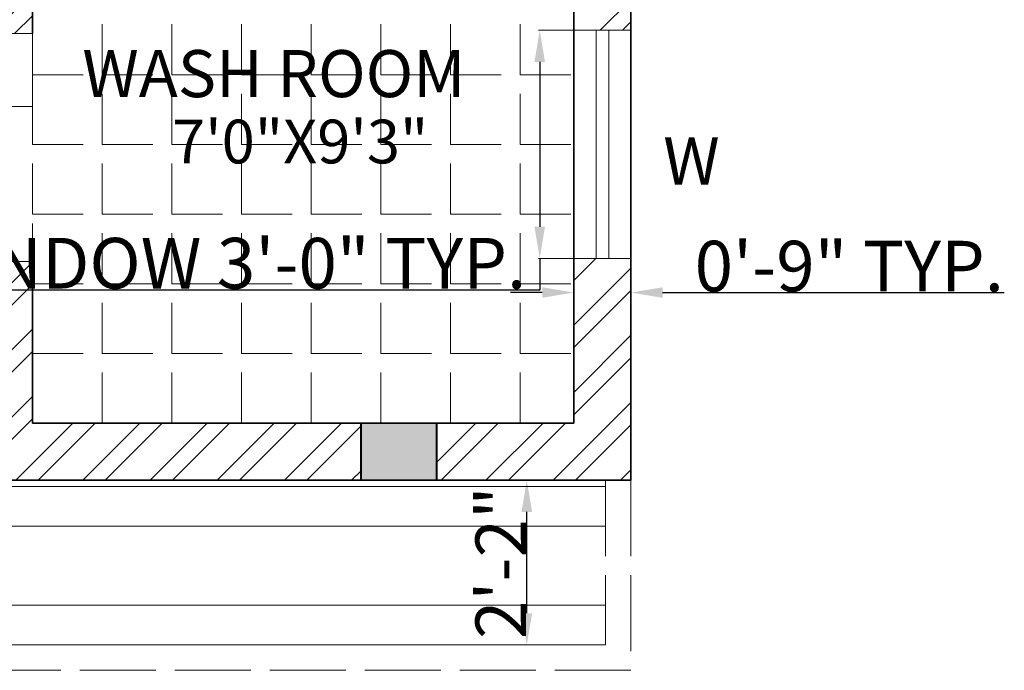
# Model space of a CAD drawing. Units: inches. Extents: x 351 to 1738, y -265 to 286.
# Tile 30 of 38: x 1470 to 1626, y -203 to -100. Entities that reach past the tile are written whole.
import ezdxf

# ---------------------------------------------------------------- set-up
doc = ezdxf.new("R2010")
doc.units = ezdxf.units.IN
doc.header["$MEASUREMENT"] = 0
doc.linetypes.add('ACAD_ISO02W100', pattern=[15, 12, -3])
doc.linetypes.add('ACAD_ISO03W100', pattern=[30, 12, -18])
for name, color, linetype, lineweight in [('A-ANNO-DIMS', 2, 'Continuous', 18), ('A-ANNO-SYMB', 7, 'Continuous', 18), ('A-AREA-IDEN', 7, 'Continuous', 18), ('A-COLS', 7, 'Continuous', 40), ('A-COLS-PATT', 6, 'Continuous', 13), ('A-DOOR', 3, 'Continuous', 18), ('A-DOOR-HIDN', 3, 'ACAD_ISO03W100', 13), ('A-FLOR-OVHD', 1, 'ACAD_ISO02W100', 18), ('A-FLOR-PATT', 9, 'Continuous', 9), ('A-GLAZ', 4, 'Continuous', 18), ('A-WALL', 7, 'Continuous', 35), ('A-WALL-PATT', 152, 'Continuous', 13)]:
    doc.layers.add(name, color=color, linetype=linetype, lineweight=lineweight)
doc.styles.add('Annotative', font='arial.ttf')
doc.styles.get("Standard").update_dxf_attribs({"font": 'arial.ttf'})
doc.dimstyles.get("Standard").update_dxf_attribs({"dimtxt": 8, "dimasz": 5, "dimexe": 0.18, "dimexo": 0.0625, "dimgap": 0.09, "dimtad": 1, "dimtoh": 1, "dimzin": 0, "dimdsep": 46, "dimlunit": 4, "dimtxsty": 'Standard', "dimcen": 0, "dimclre": 256, "dimadec": 0, "dimazin": 0, "dimtfac": 1, "dimtofl": 0, "dimtmove": 0, "dimatfit": 3, "dimfxl": 1, "dimtolj": 1, "dimtzin": 0, "dimlwe": -1, "dimarcsym": 0})

# ---------------------------------------------------------------- blocks, each defined once
blk = doc.blocks.new('*D10')
at = {"layer": 'A-ANNO-DIMS', "color": 0, "transparency": 16777216}
for p, q in [((1562.64, -173.04), (1550.08, -173.04)), ((1562.64, -199.04), (1550.08, -199.04))]:
    blk.add_line(p, q, dxfattribs=at)
at = {"layer": 'A-ANNO-DIMS', "color": 0, "lineweight": -2, "transparency": 16777216}
blk.add_line((1550.26, -194.04), (1550.26, -178.04), dxfattribs=at)
at = {"layer": 'A-ANNO-DIMS', "color": 0, "transparency": 16777216}
for points in [[(1549.43, -178.04), (1551.1, -178.04), (1550.26, -173.04)], [(1549.43, -194.04), (1551.1, -194.04), (1550.26, -199.04)]]:
    blk.add_solid(points, dxfattribs=at)
at = {"layer": 'Defpoints', "color": 0, "transparency": 16777216}
for p in [(1550.26, -173.04), (1562.7, -173.04), (1562.7, -199.04)]:
    blk.add_point(p, dxfattribs=at)
at = {"layer": 'A-ANNO-DIMS', "color": 0, "transparency": 16777216, "insert": (1546.16, -186.04), "char_height": 8, "attachment_point": 5, "rotation": 90}
blk.add_mtext('\\A1;2\'-2"', dxfattribs=at)
blk = doc.blocks.new('WIN-36')
for p, q in [((0, 5.5), (36, 5.5)), ((0, 3.5), (36, 3.5))]:
    blk.add_line(p, q)
blk.add_lwpolyline([(0, 9), (36, 9), (36, 0), (0, 0)], close=True)
blk = doc.blocks.new('*D32')
at = {"layer": 'A-ANNO-DIMS', "transparency": 16777216}
for p, q in [((1557.64, -102), (1552.12, -102)), ((1557.64, -138), (1552.12, -138))]:
    blk.add_line(p, q, dxfattribs=at)
at = {"layer": 'A-ANNO-DIMS', "color": 0, "lineweight": -2, "transparency": 16777216}
for p, q in [((1552.3, -107), (1552.3, -133)), ((1552.3, -138), (1552.3, -143)), ((1552.3, -143), (1450.98, -143))]:
    blk.add_line(p, q, dxfattribs=at)
at = {"layer": 'A-ANNO-DIMS', "color": 0, "transparency": 16777216}
for points in [[(1551.47, -107), (1553.14, -107), (1552.3, -102)], [(1551.47, -133), (1553.14, -133), (1552.3, -138)]]:
    blk.add_solid(points, dxfattribs=at)
at = {"layer": 'Defpoints', "color": 0, "transparency": 16777216}
for p in [(1557.7, -102), (1552.3, -138), (1557.7, -138)]:
    blk.add_point(p, dxfattribs=at)
at = {"layer": 'A-ANNO-DIMS', "color": 0, "transparency": 16777216, "insert": (1501.6, -138.77), "char_height": 8, "attachment_point": 5}
blk.add_mtext('\\A1;WINDOW 3\'-0" TYP.', dxfattribs=at)
blk = doc.blocks.new('*D33')
at = {"layer": 'A-ANNO-DIMS', "transparency": 16777216}
for p, q in [((1557.7, -138.06), (1557.7, -143.58)), ((1566.7, -138.06), (1566.7, -143.58))]:
    blk.add_line(p, q, dxfattribs=at)
at = {"layer": 'A-ANNO-DIMS', "color": 0, "lineweight": -2, "transparency": 16777216}
for p, q in [((1552.7, -143.4), (1547.7, -143.4)), ((1571.7, -143.4), (1625.65, -143.4))]:
    blk.add_line(p, q, dxfattribs=at)
at = {"layer": 'A-ANNO-DIMS', "color": 0, "transparency": 16777216}
for points in [[(1552.7, -142.57), (1552.7, -144.23), (1557.7, -143.4)], [(1571.7, -142.57), (1571.7, -144.23), (1566.7, -143.4)]]:
    blk.add_solid(points, dxfattribs=at)
at = {"layer": 'Defpoints', "color": 0, "transparency": 16777216}
for p in [(1557.7, -138), (1566.7, -138), (1566.7, -143.4)]:
    blk.add_point(p, dxfattribs=at)
at = {"layer": 'A-ANNO-DIMS', "color": 0, "transparency": 16777216, "insert": (1601.18, -139.23), "char_height": 8, "attachment_point": 5}
blk.add_mtext('\\A1;0\'-9" TYP.', dxfattribs=at)

msp = doc.modelspace()

# ---------------------------------------------------------------- hatches: boundary and pattern name
at = {"layer": 'A-COLS-PATT'}
h = msp.add_hatch(color=256, dxfattribs=at)
h.dxf.hatch_style = 1
h.paths.add_polyline_path([(1112.704, 237.963), (1103.704, 237.963), (1103.704, 228.963), (1112.704, 228.963)])
h.paths.add_polyline_path([(1115.704, 237.963), (1112.704, 237.963), (1112.704, 228.963), (1115.704, 228.963)])
h.paths.add_polyline_path([(1043.704, 255.963), (1034.704, 255.963), (1034.704, 243.963), (1043.704, 243.963)])
h.paths.add_polyline_path([(1043.704, 210.963), (1034.704, 210.963), (1034.704, 198.963), (1043.704, 198.963)])
h.paths.add_polyline_path([(1043.704, -45.037), (1034.704, -45.037), (1034.704, -57.037), (1043.704, -57.037)])
h.paths.add_polyline_path([(1112.704, -45.037), (1103.704, -45.037), (1103.704, -57.037), (1112.704, -57.037)])
h.paths.add_polyline_path([(1112.704, -161.037), (1103.704, -161.037), (1103.704, -164.037), (1103.704, -173.037), (1112.704, -173.037)])
h.paths.add_polyline_path([(1043.704, -161.037), (1034.704, -161.037), (1034.704, -173.037), (1043.704, -173.037)])
h.paths.add_polyline_path([(1248.549, -164.037), (1236.549, -164.037), (1236.549, -173.037), (1248.549, -173.037)])
h.paths.add_polyline_path([(1248.549, -50), (1236.549, -50), (1236.549, -59), (1248.549, -59)])
h.paths.add_polyline_path([(1248.704, 73.463), (1244.704, 73.463), (1244.704, 64.463), (1248.704, 64.463)])
h.paths.add_polyline_path([(1244.704, 73.463), (1236.704, 73.463), (1236.704, 64.463), (1244.704, 64.463)])
h.paths.add_polyline_path([(1248.704, 237.963), (1236.704, 237.963), (1236.704, 228.963), (1248.704, 228.963)])
h.paths.add_polyline_path([(1392.204, 237.963), (1380.204, 237.963), (1380.204, 228.963), (1392.204, 228.963)])
h.paths.add_polyline_path([(1536.064, 237.963), (1524.064, 237.963), (1524.064, 228.963), (1536.064, 228.963)])
h.paths.add_polyline_path([(1536.064, 73.463), (1524.064, 73.463), (1524.064, 64.463), (1536.064, 64.463)])
h.paths.add_polyline_path([(1384.204, 73.463), (1380.204, 73.463), (1380.204, 64.463), (1384.204, 64.463)])
h.paths.add_polyline_path([(1392.064, 73.463), (1384.204, 73.463), (1384.204, 64.463), (1392.064, 64.463)])
h.paths.add_polyline_path([(1536.064, -53.037), (1524.064, -53.037), (1524.064, -57.037), (1536.064, -57.037)])
h.paths.add_polyline_path([(1536.064, -48.037), (1524.064, -48.037), (1524.064, -53.037), (1536.064, -53.037)])
h.paths.add_polyline_path([(1392.064, -48.037), (1380.064, -48.037), (1380.064, -56.5), (1380.065, -57.037), (1392.064, -57.037)])
h.paths.add_polyline_path([(1536.064, -164.037), (1524.064, -164.037), (1524.064, -173.037), (1536.064, -173.037)])
at = {"layer": 'A-FLOR-PATT', "transparency": 33554559}
h = msp.add_hatch(dxfattribs=at)
h.set_pattern_fill('ANSI37', color=256, scale=200, angle=135)
h.set_pattern_definition([(180, (1112.704, -164.037), (-2e-15, -25), []), (270, (1112.704, -164.037), (25, -5e-15), [])])
h.paths.add_polyline_path([(1380.064, 73.463), (1380.132, 148.463), (1338.064, 148.463), (1290.704, 148.463), (1290.704, 88.463), (1248.704, 88.463), (1248.704, -2.009), (1244.704, -2.009), (1244.704, 142.457), (1160.704, 142.457), (1160.704, 158.963), (1160.704, 170.137), (1160.704, 206.137), (1160.704, 228.963), (1112.704, 228.963), (1112.704, 209.963), (1112.704, 168.963), (1124.704, 168.963), (1124.704, 162.963), (1112.704, 162.963), (1112.704, 64.463), (1112.704, 60.463), (1112.704, 0.463), (1112.704, -48.026), (1146.804, -47.981), (1146.804, -35.691), (1207.804, -35.691), (1207.804, -47.902), (1236.542, -47.864), (1236.544, -50.009), (1248.5, -50.009), (1248.506, -102.915), (1248.512, -150.915), (1248.514, -164.037), (1248.549, -164.037), (1273.017, -164.037), (1273.017, -128.799), (1355.24, -128.799), (1355.24, -164.037), (1384.204, -164.037), (1384.204, -57.037), (1380.064, -57.037), (1380.064, -48.037), (1392.064, -48.037), (1392.064, -53.037), (1406.549, -53.037), (1406.549, -57.037), (1401.204, -57.037), (1401.204, -147.037), (1468.204, -147.037), (1468.204, -138.5), (1472.204, -138.5), (1472.204, -102.5), (1468.204, -102.5), (1468.204, -57.037), (1442.549, -57.037), (1442.549, -53.037), (1463.049, -53.037), (1463.049, -40.747), (1524.049, -40.747), (1524.049, -48.037), (1536.064, -48.037), (1536.064, -53.037), (1557.704, -53.037), (1557.704, 204.963), (1384.204, 204.963), (1384.204, 73.463), (1392.064, 73.463), (1392.064, 64.463), (1384.204, 64.463), (1384.204, -3.5), (1380.204, -3.537), (1380.204, 64.463), (1380.064, 64.463)])
h.paths.add_polyline_path([(1510.714, 86.458, -0.1039845), (1511.661, 85.595, 0.4704384), (1510.158, 87.614, 0.0961001)], flags=16)
h.paths.add_polyline_path([(1510.443, 100.266, 0.009798), (1504.693, 100.48, 0.0287898), (1504.6, 99.767, -0.1653311), (1505.519, 96.135, -0.1436014)], flags=16)
h.paths.add_polyline_path([(1487.201, 85.595, -0.1039845), (1488.148, 86.458, 0.0961001), (1488.704, 87.614, 0.4704384)], flags=0)
h.paths.add_polyline_path([(1495.052, 100.43), (1494.178, 100.43, -0.0264629), (1494.262, 99.774, -0.1442193)], flags=16)
h.paths.add_polyline_path([(1444.485, 86.458, -0.1039845), (1445.433, 85.595, 0.4704384), (1443.93, 87.614, 0.0961001)], flags=16)
h.paths.add_polyline_path([(1420.972, 85.595, -0.1039845), (1421.92, 86.458, 0.0961001), (1422.475, 87.614, 0.4704384)], flags=16)
h.paths.add_polyline_path([(1428.632, 100.335, 0.0010541), (1427.971, 100.309, -0.0215241), (1428.033, 99.774, -0.1143008)], flags=16)
h.paths.add_polyline_path([(1419.906, 143.708, 0.0249793), (1420.222, 157.526), (1421.573, 159.101), (1421.573, 175.369), (1391.393, 175.369), (1391.393, 200.519), (1542.294, 200.519), (1542.294, 175.369), (1512.028, 175.369, 0.0198653), (1511.521, 153.838, 0.0251335), (1512.758, 118.323, 0.0205529), (1512.942, 115.253), (1419.834, 115.253, -0.0004142), (1419.843, 124.798), (1413.059, 124.798), (1413.059, 84.437, -0.0618528), (1415.831, 80.45, -0.0930773), (1420.972, 85.595, -0.2675367), (1422.371, 84.732, 0.0851103), (1424.052, 84.616, -0.8853927), (1424.033, 84.851, -1.1258145), (1424.073, 84.366, -0.0879871), (1422.371, 84.732, -0.2675367), (1422.326, 83.089, -0.3705421), (1420.972, 85.595, 0.0930773), (1415.831, 80.45, -0.0874142), (1417.914, 73.937), (1418.941, 73.937, 0.0272504), (1418.913, 76.906, -0.1157032), (1421.051, 73.937), (1445.354, 73.937, -0.1157032), (1447.492, 76.906, 0.0272504), (1447.464, 73.937), (1448.491, 73.937, -0.0874142), (1450.574, 80.45, 0.0930773), (1445.433, 85.595, -0.3705421), (1444.079, 83.089, -0.2675367), (1444.034, 84.732, -0.0879871), (1442.332, 84.366, -1.1258145), (1442.372, 84.851, -2.0327363), (1442.364, 84.368, 0.0863779), (1444.034, 84.732, -0.2675367), (1445.433, 85.595, -0.0930773), (1450.574, 80.45, -0.2577317), (1466.483, 90.927, -0.4786702), (1468.832, 91.907, -0.4786702), (1471.18, 90.927, -0.26264), (1483.053, 81.78, -0.0718662), (1487.201, 85.595, -0.2675367), (1488.6, 84.732, 0.0851103), (1490.28, 84.616, -0.8853927), (1490.262, 84.851, -1.1258145), (1490.301, 84.366, -0.0879871), (1488.6, 84.732, -0.2675367), (1488.554, 83.089, -0.3705421), (1487.201, 85.595, 0.0718662), (1483.053, 81.78, -0.1320648), (1484.143, 73.937), (1485.169, 73.937, 0.0272504), (1485.142, 76.906, -0.1157032), (1487.28, 73.937), (1511.582, 73.937, -0.1157032), (1513.72, 76.906, 0.0272504), (1513.693, 73.937), (1514.719, 73.937, -0.0874142), (1516.802, 80.45, 0.0930773), (1511.661, 85.595, -0.3705421), (1510.308, 83.089, -0.2675367), (1510.262, 84.732, -0.0879871), (1508.561, 84.366, -1.1258145), (1508.601, 84.851, -2.0327363), (1508.592, 84.368, 0.0863779), (1510.262, 84.732, -0.2675367), (1511.661, 85.595, -0.0930773), (1516.802, 80.45, -0.0618528), (1519.575, 84.437), (1519.575, 73.937), (1413.059, 73.937), (1413.059, 124.798), (1419.843, 124.798, -0.0008205)], flags=16)
h.paths.add_polyline_path([(1220.149, 54.133, -0.1039845), (1220.869, 53.476, 0.4704384), (1219.727, 55.011, 0.0961001)], flags=16)
h.paths.add_polyline_path([(1219.944, 64.626, 0.009798), (1215.574, 64.789, 0.0287898), (1215.503, 64.247, -0.1653311), (1216.201, 61.487, -0.1436014)], flags=16)
h.paths.add_polyline_path([(1209.779, 64.449, 0.0974459), (1209.339, 64.751), (1208.247, 64.751, 0.1273905), (1207.7, 64.326, 0.1715858), (1206.95, 61.475, -0.1588542), (1207.636, 59.45, 0.0158984), (1207.795, 59.218, 0.0615457), (1208.598, 59.616, 0.1754158), (1208.638, 60.099, -0.2847793), (1209.348, 62.472, 0.3262165)], flags=16)
h.paths.add_polyline_path([(1169.818, 54.133, -0.1039845), (1170.538, 53.476, 0.4704384), (1169.396, 55.011, 0.0961001)], flags=16)
h.paths.add_polyline_path([(1159.017, 62.472, 0.2847642), (1158.307, 60.099, -0.1754332), (1158.267, 59.616, 0.3929302), (1159.448, 64.449, -0.3262298)], flags=16)
h.paths.add_polyline_path([(1156.342, 58.239, -0.1783213), (1154.011, 55.31, -0.1747359), (1154.722, 55.233, -0.2008015), (1156.27, 56.086, 0.1269899), (1157.283, 58.991, -0.0912053)], flags=16)
h.paths.add_polyline_path([(1156.624, 61.413, 0.1572752), (1157.316, 64.247, 0.1696217)], flags=16)
h.paths.add_polyline_path([(1152.67, 54.133, -0.0961001), (1151.95, 53.476, 0.0640762), (1154.465, 54.384, 0.1990158)], flags=16)
h.paths.add_polyline_path([(1202.281, 53.476, -0.1039845), (1203, 54.133, 0.0961001), (1203.423, 55.011, 0.4704384)], flags=0)
h.paths.add_polyline_path([(1151.139, 97.64, 0.0249793), (1151.379, 108.141), (1152.406, 109.338), (1152.406, 121.701), (1129.47, 121.701), (1129.47, 140.814), (1244.149, 140.814), (1244.149, 121.701), (1221.148, 121.701, 0.0198653), (1220.763, 105.338, 0.0251335), (1221.703, 78.349, 0.0205529), (1221.843, 76.016), (1151.078, 76.016, -0.1287433), (1148.786, 65.037, 0.5393525), (1150.327, 64.171, -0.027594), (1163.481, 64.751, 0.0976954), (1163.04, 64.449, 0.3262165), (1163.471, 62.472, -0.2847765), (1164.181, 60.099, -0.1947567), (1165.846, 61.443, -0.1554021), (1165.172, 64.247, -0.1660224), (1165.869, 61.475, -0.1770142), (1167.852, 62.77, -0.4482027), (1169.974, 60.807, -0.3934987), (1167.679, 57.86, -0.8955483), (1168.438, 54.524, -0.3557668), (1166.218, 56.086, -0.066024), (1165.505, 57.539), (1165.251, 56.243, -0.3717324), (1164.02, 59.758, -0.3736141), (1163.04, 64.449, -0.0976954), (1163.481, 64.751, 0.0213538), (1153.294, 64.429, -0.1341826), (1156.695, 61.368, 0.1868727), (1154.636, 62.77, 0.4482027), (1152.514, 60.807, 0.4037263), (1154.905, 57.846, 0.7112192), (1153.334, 55, 0.5315397), (1151.95, 53.476, -0.2675367), (1153.013, 52.821, 0.0851103), (1154.29, 52.732, -0.8853927), (1154.276, 52.911, -1.1258145), (1154.306, 52.543, -0.0879871), (1153.013, 52.821, -0.2675367), (1152.978, 51.572, -0.3705421), (1151.95, 53.476, 0.0930773), (1148.043, 49.566, -0.0874142), (1149.626, 44.617), (1150.406, 44.617, 0.0272504), (1150.385, 46.873, -0.1157032), (1152.01, 44.617), (1170.478, 44.617, -0.1157032), (1172.103, 46.873, 0.0272504), (1172.082, 44.617), (1172.862, 44.617, -0.0874142), (1174.445, 49.566, 0.0930773), (1170.538, 53.476, -0.3705421), (1169.51, 51.572, -0.2675367), (1169.475, 52.821, -0.0879871), (1168.182, 52.543, -1.1258145), (1168.212, 52.911, -2.0327363), (1168.206, 52.544, 0.0863779), (1169.475, 52.821, -0.2675367), (1170.538, 53.476, -0.0930773), (1174.445, 49.566, -0.2577317), (1186.536, 57.528, -0.4786702), (1188.321, 58.273, -0.4786702), (1190.106, 57.528, -0.26264), (1199.128, 50.577, -0.0718662), (1202.281, 53.476, -0.2675367), (1203.344, 52.821, 0.0851103), (1204.621, 52.732, -0.8853927), (1204.607, 52.911, -1.1258145), (1204.637, 52.543, -0.0879871), (1203.344, 52.821, -0.2675367), (1203.309, 51.572, -0.3705421), (1202.281, 53.476, 0.0718662), (1199.128, 50.577, -0.1320648), (1199.957, 44.617), (1200.737, 44.617, 0.0272504), (1200.716, 46.873, -0.1157032), (1202.341, 44.617), (1220.809, 44.617, -0.1157032), (1222.434, 46.873, 0.0272504), (1222.413, 44.617), (1223.193, 44.617, -0.0874142), (1224.776, 49.566, 0.0930773), (1220.869, 53.476, -0.3705421), (1219.841, 51.572, -0.2675367), (1219.806, 52.821, -0.0879871), (1218.513, 52.543, -1.1258145), (1218.543, 52.911, -2.0327363), (1218.537, 52.544, 0.0863779), (1219.806, 52.821, -0.2675367), (1220.869, 53.476, -0.0930773), (1224.776, 49.566, -0.0618528), (1226.883, 52.597), (1226.883, 44.617), (1145.936, 44.617), (1145.936, 83.269), (1151.091, 83.269, -0.0008205)], flags=16)
h.paths.add_polyline_path([(1218.01, 57.86, -0.8955483), (1218.769, 54.524, -0.3557668), (1216.549, 56.086, -0.066024), (1215.836, 57.539), (1215.582, 56.243, -0.3717324), (1214.351, 59.758, -0.3736141), (1213.371, 64.449, 0.3262165), (1213.802, 62.472, -0.2847765), (1214.512, 60.099, -0.1947567), (1216.177, 61.443, -0.1799907), (1218.183, 62.77, -0.4482027), (1220.305, 60.807, -0.3934987)], flags=16)
h.paths.add_polyline_path([(1424.735, 91.363, -0.3934987), (1421.715, 95.241, -0.4482027), (1424.507, 97.824, -0.1799907), (1427.147, 96.077, -0.1947567), (1429.338, 94.309, -0.2847765), (1430.272, 97.432, 0.3262165), (1430.839, 100.034, -0.3736141), (1429.55, 93.861, -0.3717324), (1427.929, 89.235), (1427.596, 90.941, -0.066024), (1426.657, 89.029, -0.3557668), (1423.736, 86.973, -0.8955483)], flags=16)
h.paths.add_polyline_path([(1238.033, 131.257, -1), (1227.329, 131.257, -1)], flags=0)
h.paths.add_polyline_path([(1235.357, 131.257, -1), (1230.005, 131.257, -1)], flags=0)
h.paths.add_polyline_path([(1214.039, 54.243, 0.1543819), (1214.38, 53.992, 0.3589549), (1213.613, 54.016, 0.6039484), (1214.379, 53.657, 0.3713191), (1213.968, 52.872, 0.1879935), (1214.312, 52.809, -0.592455), (1213.953, 52.967, -0.2942791), (1214.083, 53.691, -1.3001871), (1213.881, 54.134, -0.2837621), (1214.469, 53.896, 1.1509396)], flags=16)
h.paths.add_polyline_path([(1212.091, 56.286, -0.4084338), (1211.337, 56.445, -0.0362594), (1211.098, 56.848, -0.2360976), (1211.59, 56.63, 0.0353445), (1211.835, 56.543, -0.4752408), (1212.091, 56.286, -0.4752408), (1212.438, 56.182, 0.0353445), (1212.631, 56.007, -0.2360976), (1213.056, 55.676, -0.0362594), (1212.588, 55.697, -0.4084338)], flags=16)
h.paths.add_polyline_path([(1211.469, 50.297, 0.296043), (1210.47, 50.527, 0.310883), (1211.931, 50.148, 0.0212546)], flags=16)
h.paths.add_polyline_path([(1213.739, 51.818, -0.0362594), (1213.271, 51.838, -0.4084337), (1212.774, 52.427, -0.0947856), (1212.293, 50.703, 1.1504738), (1212.911, 50.232, 0.1662877), (1213.265, 50.68, -0.0252543), (1212.603, 50.13, 1.0879317), (1212.471, 49.407, 0.1662877), (1213.02, 49.251, -0.016128), (1212.567, 49.563, -0.286859), (1212.217, 49.638, 0.0221563), (1212.046, 50.055, -0.6461302), (1212.185, 50.498, 0.0884116), (1212.732, 52.077, -1.1860374), (1213.121, 52.323, 0.0353445), (1213.314, 52.148, -0.2360976)], flags=16)
h.paths.add_polyline_path([(1212.094, 50.342, -0.0485241), (1211.54, 49.605, -1.1038339), (1211.397, 48.738, -0.7855147), (1211.683, 48.254, -0.3920429), (1210.948, 48.525, -0.3928194), (1210.561, 47.995, -0.592455), (1210.201, 48.153, -0.2942791), (1210.331, 48.877, -0.7041716), (1210.316, 49.592, -0.6793441), (1210.729, 50.112, 0.5636764)], flags=16)
h.paths.add_polyline_path([(1211.274, 49.829, -0.1398258), (1210.745, 49.859, -0.2178785), (1210.948, 49.509, -0.4985724)], flags=0)
h.paths.add_polyline_path([(1433.426, 81.49, -0.181571), (1434.245, 81.788, -0.0080665), (1433.726, 82.205, 0.0455784), (1432.755, 81.242, 0.1790113)], flags=16)
h.paths.add_polyline_path([(1434.146, 81.009, -0.1324418), (1433.645, 80.771, 0.2590893), (1433.234, 80.471, -0.1802109), (1433.392, 80.805, -0.1699398), (1432.758, 81.109, 0.0326525), (1433.273, 80.474, -0.4933627), (1434.046, 80.146, -0.3904966)], flags=16)
h.paths.add_polyline_path([(1434.83, 80.047, -0.9475376), (1435.294, 79.576, -0.2991282), (1434.625, 79.404, -0.2704392), (1435.01, 78.591, -0.592455), (1434.537, 78.382, -0.3928194), (1434.027, 79.08, -0.3920429), (1433.06, 78.723, -0.3520423), (1433.003, 79.197, -0.1972159), (1433.75, 79.734, -0.7136405), (1434.447, 79.939, -0.2147903), (1434.819, 80.475, 0.4088333), (1435.075, 80.803, -0.2261519)], flags=16)
h.paths.add_polyline_path([(1432.67, 81.217, -0.4542182), (1431.897, 79.923, -0.4144105), (1431.301, 80.035, 0.0161291), (1431.897, 80.445, 0.2795702), (1432.073, 80.871, -0.2895037), (1431.103, 81.321, -0.4144105), (1430.978, 81.915, 0.0161296), (1431.586, 81.521, 0.341293), (1432.125, 81.583, -0.8131856)], flags=16)
h.paths.add_polyline_path([(1429.893, 86.381, -0.9475376), (1430.358, 85.91, -0.1731062), (1429.984, 85.712, -0.0388172), (1431.625, 84.214, -0.0879005), (1432.097, 88.549, -0.0497684), (1431.254, 88.49, -0.2360976), (1431.814, 88.925, 0.0353445), (1432.067, 89.155, -0.4752408), (1432.524, 89.291, -0.4752408), (1432.86, 89.63, 0.0353445), (1433.182, 89.744, -0.2360976), (1433.83, 90.032, -0.0362594), (1433.516, 89.502, -0.4084338), (1432.524, 89.291, -0.3124239), (1432.106, 88.58, 0.0885594), (1431.625, 84.214, -0.4084337), (1430.971, 83.439, -0.0362594), (1430.355, 83.412, -0.2360976), (1430.914, 83.847, 0.0353445), (1431.168, 84.078, -0.4752408), (1431.625, 84.214, 0.0388172), (1429.984, 85.712, -0.3217316), (1429.333, 86.048, -0.32743), (1429.883, 86.809, 0.4088333), (1430.138, 87.138, -0.2261519)], flags=16)
h.paths.add_polyline_path([(1211.206, 58.616, -0.9997836), (1211.336, 59.323, -0.6149935)], flags=16)
h.paths.add_polyline_path([(1210.288, 49.429, 0.1543819), (1210.629, 49.178, 0.3589549), (1209.861, 49.202, 0.6039484), (1210.627, 48.843, -0.5348247), (1210.806, 49.295, 0.7483464)], flags=16)
h.paths.add_polyline_path([(1209.589, 51.828, -0.0087906), (1209.775, 51.753, 0.1122315), (1209.466, 52.019, 1.4188509), (1209.014, 51.708, -0.4587257), (1208.651, 51.073, -0.592455), (1208.291, 51.232, -0.2942791), (1208.421, 51.955, -1.3001871), (1208.219, 52.398, -0.2260052), (1208.719, 52.257, -0.4755189), (1209.158, 52.369, -1.4554994), (1209.603, 52.664, 0.4213049), (1209.191, 52.262, -0.5912116), (1208.979, 51.796, 0.4973986), (1209.773, 51.333, 0.6493116)], flags=16)
h.paths.add_polyline_path([(1208.029, 52.041, 0.5446671), (1208.832, 52.045, 0.220132)], flags=0)
h.paths.add_polyline_path([(1210.438, 51.425, -0.2041997), (1210.277, 52.018, 0.2708262), (1209.915, 52.897, 0.3241145)], flags=0)
h.paths.add_polyline_path([(1209.668, 52.407, -0.60139), (1208.99, 52.221, -0.3949159), (1208.248, 52.83, -0.8367916), (1208.651, 53.017, -0.3384876), (1209.039, 52.571, 0.1941379), (1209.191, 52.262, 0.4139945), (1209.712, 52.475, 0.5177103), (1210.503, 51.416, 0.401922), (1209.493, 50.93, 0.2063956), (1209.516, 50.165, -0.3194629), (1210.417, 51.418, -0.466635)], flags=16)
h.paths.add_polyline_path([(1206.601, 56.086, -0.3557668), (1204.381, 54.524, -0.9211983), (1205.236, 57.846, 0.2065693), (1207.614, 58.991, -0.1269899)], flags=16)
h.paths.add_polyline_path([(1435.487, 82.816, 0.5277653), (1436.615, 83.361, 0.5085402), (1437.05, 82.433, 0.592455), (1437.524, 82.641, 0.3312448), (1436.963, 83.548, 0.3878632), (1437.808, 83.626, 0.5929544), (1437.618, 84.176, 0.2260158), (1436.961, 83.99, 0.3182053), (1437.588, 84.854, 0.6893744), (1437.05, 84.991, 0.3357648), (1436.539, 84.41, -0.1569934), (1436.404, 84.065, -0.4346112), (1436.961, 83.99, -0.2147903), (1437.333, 84.526, 0.4088333), (1437.588, 84.854, -0.2261519), (1437.343, 84.097, -0.9475376), (1437.808, 83.626, -0.2991282), (1437.139, 83.455, -0.2704392), (1437.524, 82.641, -0.592455), (1437.05, 82.433, -0.3928194), (1436.541, 83.13, -0.4396601), (1435.475, 82.794, -0.174614), (1435.942, 82.244, -0.2063956), (1435.912, 81.237, -0.2708262), (1435.125, 82.208, 0.2079765), (1434.686, 82.904, -0.1964955)], flags=16)
h.paths.add_polyline_path([(1435.386, 84.832, 0.270811), (1434.91, 83.676, -0.2042174), (1434.699, 82.895, 0.3241145)], flags=0)
h.paths.add_polyline_path([(1435.68, 84.18, -0.2176564), (1435.554, 83.304, -0.1767045), (1436.236, 83.778, -0.3730364)], flags=0)
h.paths.add_polyline_path([(1435.566, 100.034, 0.3262165), (1436.133, 97.432, -0.2847765), (1437.067, 94.309, -0.1947567), (1439.258, 96.077, -0.1554021), (1438.371, 99.767, -0.1660224), (1439.289, 96.12, -0.1770142), (1441.897, 97.824, -0.4482027), (1444.69, 95.241, -0.3934987), (1441.67, 91.363, -0.8955483), (1442.669, 86.973, -0.3557668), (1439.748, 89.029, -0.066024), (1438.809, 90.941), (1438.476, 89.235, -0.3717324), (1436.855, 93.861, -0.3736141)], flags=16)
h.paths.add_polyline_path([(1191.252, 49.507, -0.2740221), (1190.658, 48.409, 0.2675367), (1191.311, 47.344, 0.3705421)], flags=0)
h.paths.add_polyline_path([(1190.301, 49.717, 0.1990158), (1188.619, 49.04, 0.0640762), (1191.252, 49.507, -0.0961001)], flags=0)
h.paths.add_polyline_path([(1189.518, 47.857, 1.1258145), (1189.676, 47.523, 2.0446052)], flags=0)
h.paths.add_polyline_path([(1464.974, 80.372, 0.2740221), (1465.756, 78.927, -0.0830131)], flags=0)
h.paths.add_polyline_path([(1464.974, 80.372, 0.3705421), (1464.897, 77.525, 0.5763244)], flags=0)
h.paths.add_polyline_path([(1464.974, 80.372, -0.4704384), (1467.284, 81.372, -0.0961001), (1466.226, 80.648, -0.1990158), (1468.439, 79.757, -0.0640762)], flags=0)
h.paths.add_polyline_path([(1189.511, 56.43, -0.2594668), (1188.321, 56.391, -0.2594668), (1187.13, 56.43, 0.0851103), (1188.193, 55.716, -0.8853927), (1188.27, 55.878, -1.1960133), (1188.355, 55.442, 0.1014587)], flags=0)
h.paths.add_polyline_path([(1188.321, 57.596, 0.0780722), (1187.678, 57.24, 0.0155503), (1188.321, 57.136, 0.0155503), (1188.964, 57.24, 0.0780722)], flags=0)
h.paths.add_polyline_path([(1190.164, 55.365, -0.5763244), (1190.106, 57.528, -0.1982945), (1188.321, 58.319, -0.1982945), (1186.536, 57.528, -0.5763244), (1186.477, 55.365, -0.3705421), (1186.536, 57.528, 0.1982945), (1188.321, 58.319, 0.1982945), (1190.106, 57.528, -0.3705421)], flags=0)
h.paths.add_polyline_path([(1188.372, 55.878, 1.1258145), (1188.529, 55.544, 2.0446052)], flags=0)
h.paths.add_polyline_path([(1186.341, 49.717, -0.0961001), (1185.389, 49.507, 0.0640762), (1188.022, 49.04, 0.1990158)], flags=0)
h.paths.add_polyline_path([(1185.389, 49.507, -0.2675367), (1185.984, 48.409, 0.0851103), (1187.046, 47.695, -0.8853927), (1187.123, 47.857, -1.1258145), (1186.966, 47.523, -0.0879871), (1185.984, 48.409, -0.2675367), (1185.331, 47.344, -0.3705421)], flags=0)
h.paths.add_polyline_path([(1399.441, 187.944, -1), (1413.525, 187.944, -1)], flags=0)
h.paths.add_polyline_path([(1402.962, 187.944, -1), (1410.004, 187.944, -1)], flags=0)
h.paths.add_polyline_path([(1357.663, -72.245), (1377.272, -72.245), (1377.272, -91.854), (1357.663, -91.854)], flags=16)
h.paths.add_polyline_path([(1467.256, 78.201, -1.1258145), (1467.049, 77.761, -2.0446052)], flags=0)
h.paths.add_polyline_path([(1468.822, 88.714, 0.9411249), (1469.106, 88.316, 1.1371523), (1468.765, 88.755, 0.890986), (1468.99, 88.245, 0.0948283), (1470.398, 89.481, -0.2675367), (1471.18, 90.927, -0.0281232), (1469.678, 90.547, -0.0287737), (1469.948, 90.311, -0.0203267), (1468.832, 90.41, -0.0203267), (1467.716, 90.311, -0.0287737), (1467.986, 90.547, -0.0281232), (1466.483, 90.927, -0.2675367), (1467.265, 89.481, 0.0851103), (1468.663, 88.542, -1.2023159)], flags=0)
h.paths.add_polyline_path([(1178.25, 124.523, -0.1199286), (1165.65, 124.145, -0.1073492), (1159.133, 124.446, -0.1028906), (1159.132, 130.465, -0.0748968), (1158.993, 137.956, 0.002027), (1167.844, 137.479, -0.07553), (1180.337, 137.666, -0.0758613), (1186.502, 137.688, -0.1409896), (1186.272, 130.046, -0.0954805), (1186.729, 124.748, -0.10603)], flags=0)
h.paths.add_polyline_path([(1469.225, 79.757, -0.1990158), (1471.437, 80.648, -0.0961001), (1470.379, 81.372, -0.4704384), (1472.689, 80.372, -0.3705421), (1472.766, 77.525, -0.2675367), (1471.907, 78.927, -0.0879863), (1470.615, 77.761, -1.1258491), (1470.408, 78.201, -2.0327363), (1470.642, 77.778, 0.0863779), (1471.907, 78.927, -0.2675367), (1472.689, 80.372, -0.0640762)], flags=0)
h.paths.add_polyline_path([(1430.423, 186.902, -0.0748968), (1430.24, 196.758, 0.002027), (1441.887, 196.131, -0.07553), (1458.326, 196.377, -0.0758613), (1466.438, 196.406, -0.1409896), (1466.136, 186.35, -0.0954805), (1466.737, 179.378, -0.10603), (1455.58, 179.082, -0.1199286), (1439, 178.585, -0.1073492), (1430.425, 178.981, -0.1028906)], flags=0)
h.paths.add_polyline_path([(1162.258, 49.939, 0.3357645), (1161.87, 49.497, -0.1569936), (1161.767, 49.235, -0.4346112), (1162.19, 49.178, -0.2147903), (1162.473, 49.585, 1.5291948)], flags=16)
h.paths.add_polyline_path([(1161.683, 49.021, 0.5815181), (1161.268, 49.583, 0.5927609)], flags=16)
h.paths.add_polyline_path([(1162.602, 48.058, 0.3713191), (1162.192, 48.843, 0.4345332), (1162.88, 48.962, 0.1850806), (1162.197, 48.926, 1.1218369)], flags=16)
h.paths.add_polyline_path([(1161.443, 48.941, -1.3071038), (1161.495, 48.571, -0.2177521), (1161.136, 48.254, 0.6973029), (1161.871, 49.048, 0.1215141)], flags=16)
h.paths.add_polyline_path([(1162.531, 49.429, -0.2070837), (1162.05, 49.146, -0.9920299)], flags=16)
h.paths.add_polyline_path([(1161.304, 49.578, -0.7196675), (1161.513, 50.079, -0.1304275), (1160.836, 50.168, 0.0395926)], flags=0)
h.paths.add_polyline_path([(1162.036, 50.584, -0.0080665), (1161.642, 50.9, 0.0293675), (1161.35, 50.297, -0.2057884)], flags=16)
h.paths.add_polyline_path([(1162.882, 51.392, -0.1247327), (1162.763, 51.828, -0.1011907), (1162.399, 51.438, -0.153425)], flags=0)
h.paths.add_polyline_path([(1164.235, 51.85, -0.3091075), (1164.513, 51.136, -0.6271245), (1163.781, 51.603, -0.6859091), (1162.777, 51.219, -0.2332851), (1163.303, 50.165, -0.2708262), (1162.705, 50.903, 0.2041997), (1162.381, 51.425, 0.204182), (1162.542, 52.018, -0.2708414), (1162.903, 52.897, -0.1272607), (1163.219, 52.529, -1.1686811), (1163.781, 52.587, -0.3291117), (1164.168, 53.017, -0.8367917), (1164.571, 52.83, -0.1933406), (1164.391, 52.338, -0.9475376), (1164.744, 51.981, -0.2991282)], flags=16)
h.paths.add_polyline_path([(1163.598, 51.937, -1.2629561), (1163.236, 51.831, 0.0125754), (1162.971, 51.721, 0.2306566), (1163.151, 52.407, -0.1648982), (1163.178, 52.661, -0.4493201), (1163.628, 52.262, -0.721477), (1164.154, 52.088, -0.8499982)], flags=0)
h.paths.add_polyline_path([(1161.613, 58.616, -0.9804131), (1161.525, 59.049, -2.9089348)], flags=16)
h.paths.add_polyline_path([(1160.252, 49.166, -0.4144105), (1159.799, 49.251, 0.0161291), (1160.252, 49.563, 0.2795702), (1160.386, 49.887, -0.2895037), (1159.649, 50.229, -0.4144105), (1159.554, 50.68, 0.0161296), (1160.015, 50.381, 0.6178854), (1160.526, 50.703, -0.0947856), (1160.045, 52.427, -0.1404436), (1159.682, 52.042, -0.0578559), (1159.3, 51.872, 0.5448433), (1160.046, 52.419, -0.0881216), (1160.404, 55.721, -0.0497684), (1159.763, 55.676, -0.2360976), (1160.188, 56.007, 0.0353445), (1160.381, 56.182, -0.4752408), (1160.728, 56.286, -0.4752408), (1160.984, 56.543, 0.0353445), (1161.229, 56.63, -0.2360976), (1161.721, 56.848, -0.0362594), (1161.482, 56.445, -0.4084338), (1160.728, 56.286, -0.3124239), (1160.411, 55.745, 0.0885594), (1160.045, 52.427, 0.1070813), (1160.634, 50.498, -0.4947977), (1160.839, 50.149, -0.4542182)], flags=16)
h.paths.add_polyline_path([(1160.666, 49.808, -2.0765276), (1160.828, 50.172, 0.0195861)], flags=0)
h.paths.add_polyline_path([(1158.439, 53.992, 0.1543819), (1158.78, 54.243, 0.7483463), (1158.262, 54.109, -0.3382251), (1158.492, 53.839, -0.1708158), (1159.124, 53.779, 0.4957286), (1158.938, 54.134, 0.2260157)], flags=16)
h.paths.add_polyline_path([(1160.045, 52.427, 0.0388172), (1158.798, 53.565, -0.1198178), (1158.574, 53.586, -0.3091075), (1158.851, 52.872, -0.1879935), (1158.506, 52.809, 0.592455), (1158.866, 52.967, 0.3312448), (1158.44, 53.657, 0.2012451), (1158.798, 53.565, -0.034023), (1159.901, 52.578, -0.0442527), (1159.698, 52.323, -0.4752408)], flags=16)
h.paths.add_polyline_path([(1336.926, -95.392), (1336.926, -117.945), (1291.82, -117.945), (1291.82, -95.392)], flags=16)
h.paths.add_polyline_path([(1357.535, -97.244), (1357.726, -96.697, 0.0348443)], flags=16)
h.paths.add_polyline_path([(1376.693, -96.478), (1377.301, -96.5, 0.0314968), (1375.907, -96.424), (1357.726, -96.424)], flags=16)
h.paths.add_polyline_path([(1379.403, -119.667, 0.0267056), (1380.043, -119.439, -0.0152991)], flags=16)
h.paths.add_polyline_path([(1357.726, -120.202), (1357.821, -120.202), (1357.821, -120.201)], flags=16)
h.paths.add_polyline_path([(1354.171, -104.592), (1354.469, -98.672, 0.0111377)], flags=16)
h.paths.add_polyline_path([(1355.058, -119.136), (1354.578, -118.539, 0.1431635)], flags=16)
h.paths.add_polyline_path([(1378.851, -96.821), (1378.85, -96.82), (1378.85, -96.82, -0.0496798), (1380.055, -97.191), (1378.85, -96.82, 0.1500541), (1375.135, -97.188), (1375.136, -119.44, -0.0099698), (1374.747, -116.649), (1357.726, -116.649, 0.1693849), (1357.535, -119.382), (1357.535, -119.382), (1357.535, -119.382, 0.0348176), (1357.726, -119.928), (1357.726, -119.928), (1357.726, -119.929, -0.0348772), (1357.535, -119.382), (1355.507, -119.382), (1355.317, -119.278), (1357.535, -119.382, -0.1693939), (1357.726, -116.649, -0.0391513), (1374.686, -116.113, -0.0020149), (1374.625, -115.546, 0.1153223), (1369.915, -115.474, 0.0609215), (1369.922, -101.154, 0.1151459), (1374.625, -101.079, -0.0020164), (1374.686, -100.513, -0.0391511), (1357.726, -99.977), (1374.747, -99.977, -0.0099633), (1375.135, -97.188), (1375.135, -97.188, -0.1501081)], flags=16)
h.paths.add_polyline_path([(1490.963, 91.363, -0.3934987), (1487.944, 95.241, -0.4482027), (1490.736, 97.824, -0.1799907), (1493.376, 96.077, -0.1947567), (1495.567, 94.309, -0.2847765), (1496.501, 97.432, 0.3262165), (1497.068, 100.034, -0.3736141), (1495.778, 93.861, -0.3717324), (1494.158, 89.235), (1493.824, 90.941, -0.066024), (1492.886, 89.029, -0.3557668), (1489.964, 86.973, -0.8955483)], flags=16)
h.paths.add_polyline_path([(1354.86, -97.658), (1355.316, -97.348, 0.1019112)], flags=16)
h.paths.add_polyline_path([(1497.063, 83.327, 0.1767244), (1496.37, 83.785, -0.4051388), (1496.016, 83.384, 0.4973986), (1497.06, 82.774, 0.6493116), (1496.818, 83.426, -0.0087906)], flags=16)
h.paths.add_polyline_path([(1496.339, 83.783, 0.5927609), (1496.886, 84.522, 0.5815181)], flags=16)
h.paths.add_polyline_path([(1495.11, 82.641, 0.592455), (1495.583, 82.433, 0.6769152), (1495.805, 83.59, 0.3756693)], flags=16)
h.paths.add_polyline_path([(1495.015, 84.176, -0.145057), (1495.301, 84.526, -0.4088333), (1495.045, 84.854, 0.2206292), (1495.381, 84.152, -0.199594), (1495.851, 83.764, -0.5240172), (1494.826, 83.626, -0.5929976)], flags=16)
h.paths.add_polyline_path([(1501.655, 81.915, -0.0161291), (1501.048, 81.521, -0.3927187), (1500.462, 81.37, -0.2106699), (1500.607, 81.142, 0.3066994)], flags=16)
h.paths.add_polyline_path([(1500.11, 89.291, -0.4084338), (1499.118, 89.502, -0.0362594), (1498.803, 90.032, -0.2360976), (1499.451, 89.744, 0.0353445), (1499.774, 89.63, -0.4752408), (1500.11, 89.291, -0.4752408), (1500.567, 89.155, 0.0353445), (1500.82, 88.925, -0.2360976), (1501.379, 88.49, -0.0362594), (1500.763, 88.516, -0.4084338)], flags=16)
h.paths.add_polyline_path([(1498.908, 82.205, -0.0513217), (1500.013, 81.134, -0.5879306), (1500.234, 81.676, 0.1070813), (1501.009, 84.214, -0.03529)], flags=16)
h.paths.add_polyline_path([(1496.93, 83.875, -0.2063956), (1497.247, 84.832, -0.2708262), (1497.724, 83.676, 0.2079765), (1497.944, 82.884, -0.3814554)], flags=16)
h.paths.add_polyline_path([(1496.721, 81.237, 0.2708125), (1497.509, 82.208, -0.2042157), (1497.935, 82.895, 0.3241145)], flags=16)
h.paths.add_polyline_path([(1497.529, 80.125, -0.145057), (1497.814, 80.475, -0.703182), (1498.282, 81.178, -0.1229248), (1497.977, 81.714, -0.2708368), (1499.207, 81.49, 0.2079641), (1499.993, 81.248, -0.2651454), (1499.278, 80.472, 0.3819006), (1498.808, 79.947, -0.3059049), (1498.848, 79.519, 0.4994816), (1498.574, 79.217, -0.4587257), (1498.097, 78.382, -0.592455), (1497.624, 78.591, -0.2704392), (1498.009, 79.404, -0.299116), (1497.34, 79.576, -0.5930157)], flags=16)
h.paths.add_polyline_path([(1500.736, 79.923, 0.4144105), (1501.333, 80.035, -0.3216484), (1500.192, 80.765, 0.0198856), (1499.976, 81.251, 0.4653307)], flags=16)
h.paths.add_polyline_path([(1501.009, 84.214, -0.0388172), (1502.649, 85.712, -0.1730946), (1502.276, 85.91, -0.5930157), (1502.465, 86.46, -0.145057), (1502.751, 86.809, -0.4088333), (1502.495, 87.138, 0.2206292), (1502.831, 86.436, -0.199594), (1503.301, 86.048, -0.3217316), (1502.649, 85.712, 0.0388172), (1501.009, 84.214, 0.1224486), (1501.412, 83.755, 0.4754908), (1501.335, 84.226, 0.055822), (1501.719, 83.847, -0.2360976), (1502.278, 83.412, -0.0362594), (1501.663, 83.439, -0.4084338)], flags=16)
h.paths.add_polyline_path([(1501.794, 100.034, 0.3262165), (1502.362, 97.432, -0.2847765), (1503.295, 94.309, -0.1947567), (1505.486, 96.077, -0.1799907), (1508.126, 97.824, -0.4482027), (1510.918, 95.241, -0.3934987), (1507.899, 91.363, -0.8955483), (1508.898, 86.973, -0.3557668), (1505.976, 89.029, -0.066024), (1505.038, 90.941), (1504.704, 89.235, -0.3717324), (1503.084, 93.861, -0.3736141)], flags=16)
h.paths.add_polyline_path([(1146.29, 131.257, -1), (1135.587, 131.257, -1)], flags=0)
h.paths.add_polyline_path([(1143.614, 131.257, -1), (1138.262, 131.257, -1)], flags=0)
h.paths.add_polyline_path([(1524.064, 73.463), (1536.064, 73.463), (1536.064, 64.463), (1524.064, 64.463)], flags=16)
h.paths.add_polyline_path([(1520.162, 187.944, -1), (1534.246, 187.944, -1)], flags=0)
h.paths.add_polyline_path([(1530.725, 187.944), (1527.204, 187.944), (1527.204, 184.423, 0.4142136)], flags=0)
h.paths.add_polyline_path([(1278.415, -91.154), (1331.067, -91.154), (1331.067, -80.583), (1278.415, -80.583)], flags=24)
h.paths.add_polyline_path([(1266.655, -79.354), (1354.738, -79.354), (1354.738, -67.817), (1266.655, -67.817)], flags=24)
h.paths.add_polyline_path([(1115.482, 206.184), (1155.098, 206.184), (1155.098, 217.714), (1115.482, 217.714)], flags=24)
h.paths.add_polyline_path([(1161.771, 8.501), (1222.466, 8.501), (1222.466, 19.079), (1161.771, 19.079)], flags=24)
h.paths.add_polyline_path([(1164.656, 18.795), (1210.615, 18.795), (1210.615, 30.324), (1164.656, 30.324)], flags=24)
h.paths.add_polyline_path([(1368.147, -32.882), (1379.362, -32.882), (1379.362, -21.733), (1368.147, -21.733)], flags=24)
h.paths.add_polyline_path([(1244.842, -31.012), (1256.057, -31.012), (1256.057, -19.863), (1244.842, -19.863)], flags=24)
h.paths.add_polyline_path([(1114.589, 195.739), (1156.517, 195.739), (1156.517, 206.31), (1114.589, 206.31)], flags=24)
h.paths.add_polyline_path([(1436.398, 37.632), (1505.131, 37.632), (1505.131, 48.203), (1436.398, 48.203)], flags=24)
h.paths.add_polyline_path([(1435.991, 47.919), (1507.906, 47.919), (1507.906, 59.456), (1435.991, 59.456)], flags=24)
h.paths.add_polyline_path([(1415.107, -124.896), (1457.038, -124.896), (1457.038, -114.318), (1415.107, -114.318)], flags=24)
h.paths.add_polyline_path([(1417.992, -114.602), (1457.609, -114.602), (1457.609, -103.073), (1417.992, -103.073)], flags=24)
h = msp.add_hatch(dxfattribs=at)
h.set_pattern_fill('ANSI32', color=256, scale=50, angle=135)
h.set_pattern_definition([(180, (1038.704, -199.037), (-2e-15, -18.75), []), (180, (1032.454, -192.787), (-2e-15, -18.75), [])])
h.paths.add_polyline_path([(1248.506, -102.915), (1236.559, -102.916), (1236.553, -56.864), (1112.704, -57.026), (1112.704, -57.037), (1103.704, -57.037), (1103.704, -45.037), (1103.704, 98.963), (1076.434, 98.963), (1076.549, -81.037), (1071.549, -81.037), (1043.704, -81.037), (1038.704, -81.037), (1038.704, -161.037), (1043.704, -161.037), (1043.704, -173.037), (1038.704, -173.037), (1038.704, -199.037), (1562.704, -199.037), (1562.704, -173.037), (1236.549, -173.037), (1236.549, -164.037), (1236.693, -164.037), (1236.676, -150.916), (1248.512, -150.915)])
h.paths.add_polyline_path([(1236.133, -134.078), (1247.348, -134.078), (1247.348, -122.929), (1236.133, -122.929)], flags=24)
h.paths.add_polyline_path([(1308.144, -185.548), (1321.66, -185.548), (1321.66, -174.4), (1308.144, -174.4)], flags=24)
h.paths.add_polyline_path([(1121.632, -122.88), (1179.647, -122.88), (1179.647, -112.309), (1121.632, -112.309)], flags=24)
h.paths.add_polyline_path([(1124.515, -112.593), (1177.986, -112.593), (1177.986, -101.056), (1124.515, -101.056)], flags=24)
h.paths.add_polyline_path([(1091.374, 23.58), (1104.89, 23.58), (1104.89, 34.728), (1091.374, 34.728)], flags=24)
at = {"layer": 'A-FLOR-PATT', "transparency": 33554610}
h = msp.add_hatch(dxfattribs=at)
h.set_pattern_fill('ANGLE', color=256, scale=40)
h.set_pattern_definition([(0, (1472.204, -164.037), (0, 11), [8, -3]), (90, (1472.204, -164.037), (-11, 7e-16), [8, -3])])
h.paths.add_polyline_path([(1557.704, -57.037), (1472.204, -57.037), (1472.204, -102.5), (1472.204, -138.5), (1472.204, -164.037), (1557.704, -164.037)])
at = {"layer": 'A-WALL-PATT'}
h = msp.add_hatch(dxfattribs=at)
h.set_pattern_fill('ANSI32', color=256, scale=20)
h.set_pattern_definition([(45, (1034.704, -173.037), (-5.3033, 5.3033), []), (45, (1038.24, -173.037), (-5.3033, 5.3033), [])])
h.paths.add_polyline_path([(1043.704, -57.037), (1034.704, -57.037), (1034.704, -81.037), (1043.704, -81.037)])
h.paths.add_polyline_path([(1043.704, 198.963), (1034.704, 198.963), (1034.704, -45.037), (1043.704, -45.037)])
h.paths.add_polyline_path([(1043.704, 243.963), (1034.704, 243.963), (1034.704, 237.963), (1034.704, 210.963), (1043.704, 210.963)])
h.paths.add_polyline_path([(1112.704, 255.963), (1043.704, 255.963), (1043.704, 246.963), (1103.704, 246.963), (1103.704, 237.963), (1112.704, 237.963), (1112.704, 251.963)])
h.paths.add_polyline_path([(1056.704, 207.963), (1043.704, 207.963), (1043.704, 198.963), (1056.704, 198.963)])
h.paths.add_polyline_path([(1103.704, 207.963), (1092.704, 207.963), (1092.704, 198.963), (1103.704, 198.963)])
h.paths.add_polyline_path([(1112.704, 228.963), (1103.704, 228.963), (1103.704, 74.963), (1112.704, 74.963), (1112.704, 97.5)])
h.paths.add_polyline_path([(1284.129, -164.037), (1248.549, -164.037), (1248.549, -173.037), (1284.129, -173.037)])
h.paths.add_polyline_path([(1524.064, -164.037), (1472.204, -164.037), (1472.204, -138.5), (1468.204, -138.5), (1468.204, -164.037), (1344.129, -164.037), (1344.129, -173.037), (1524.064, -173.037)])
h.paths.add_polyline_path([(1384.204, -57.037), (1380.065, -57.037), (1380.204, -164.037), (1384.204, -164.037)])
h.paths.add_polyline_path([(1566.704, -138), (1557.704, -138), (1557.704, -164.037), (1536.064, -164.037), (1536.064, -173.037), (1566.704, -173.037)])
h.paths.add_polyline_path([(1566.704, -30.189), (1557.704, -30.189), (1557.704, -53.037), (1536.064, -53.037), (1536.064, -57.037), (1557.704, -57.037), (1557.704, -102), (1566.704, -102)])
h.paths.add_polyline_path([(1524.064, -53.037), (1442.549, -53.037), (1442.549, -57.037), (1468.204, -57.037), (1468.204, -102.5), (1472.204, -102.5), (1472.204, -57.037), (1524.064, -57.037)])
h.paths.add_polyline_path([(1566.704, 120.993), (1557.704, 120.993), (1557.704, 29.811), (1566.704, 29.811)])
h.paths.add_polyline_path([(1384.204, 64.463), (1380.204, 64.463), (1380.204, -3.5), (1384.204, -3.5)])
h.paths.add_polyline_path([(1266.549, 237.963), (1248.704, 237.963), (1248.704, 228.963), (1266.549, 228.963)])
h.paths.add_polyline_path([(1329.549, 237.963), (1302.549, 237.963), (1302.549, 228.963), (1329.549, 228.963)])
h.paths.add_polyline_path([(1380.204, 237.963), (1365.549, 237.963), (1365.549, 228.963), (1380.204, 228.963)])
h.paths.add_polyline_path([(1524.064, 237.963), (1392.204, 237.963), (1392.204, 228.963), (1524.064, 228.963)])
h.paths.add_polyline_path([(1384.204, 228.963), (1380.204, 228.963), (1380.204, 73.463), (1384.204, 73.463)])
h.paths.add_polyline_path([(1566.704, 237.963), (1536.064, 237.963), (1536.064, 228.963), (1557.704, 228.963), (1557.704, 180.993), (1566.704, 180.993)])

# ---------------------------------------------------------------- linework, layer by layer
at = {"layer": 'A-COLS'}
for points in [[(1524.064, -164.037), (1524.064, -173.037)], [(1536.064, -173.037), (1536.064, -164.037)]]:
    msp.add_lwpolyline(points, dxfattribs=at)
at = {"layer": 'A-DOOR'}
for points in [[(1472.204, -102.5), (1468.204, -102.5)], [(1468.204, -138.5), (1472.204, -138.5)]]:
    msp.add_lwpolyline(points, dxfattribs=at)
at = {"layer": 'A-DOOR-HIDN'}
msp.add_line((1472.204, -102.5), (1472.204, -138.5), dxfattribs=at)
at = {"layer": 'A-FLOR-OVHD'}
for p, q in [((1562.704, -173.037), (1562.704, -199.037)), ((1566.704, -173.037), (1566.704, -203.037)), ((1562.704, -199.037), (1038.704, -199.037)), ((1566.704, -203.037), (1034.704, -203.037))]:
    msp.add_line(p, q, dxfattribs=at)
at = {"layer": 'A-WALL'}
for p, q in [((1566.704, -173.037), (1566.704, 237.963)), ((1472.204, -57.037), (1472.204, -102.5)), ((1557.704, -164.037), (1557.704, -57.037)), ((1472.204, -138.5), (1472.204, -164.037)), ((1472.204, -164.037), (1557.704, -164.037)), ((1236.549, -173.037), (1566.704, -173.037))]:
    msp.add_line(p, q, dxfattribs=at)

# ---------------------------------------------------------------- block references
at = {"layer": 'A-GLAZ', "rotation": 270.0000000000001}
msp.add_blockref('WIN-36', (1557.704, -102), dxfattribs=at)

# ---------------------------------------------------------------- texts
at = {"layer": 'A-ANNO-SYMB', "style": 'Annotative'}
msp.add_text('W', height=7.433, dxfattribs=at).set_placement((1571.805, -126.346))
at = {"layer": 'A-AREA-IDEN', "style": 'Annotative'}
for s, height, p in [('WASH ROOM', 7.4326, (1480.099, -112.554)), ('7\'0"X9\'3"', 6.9014, (1494.252, -123.011))]:
    msp.add_text(s, height=height, dxfattribs=at).set_placement(p)

# ---------------------------------------------------------------- dimensions: what is measured, and where the dimension line sits
at = {"layer": 'A-ANNO-DIMS'}
dim = msp.add_linear_dim(base=(1552.304, -138), p1=(1557.704, -102), p2=(1557.704, -138), angle=270, text='WINDOW <> TYP.', dimstyle='Standard', override={"dimdec": 1, "dimlfac": 1, "dimrnd": 0, "dimzin": 1, "dimdsep": 46, "dimlunit": 4, "dimfrac": 2}, dxfattribs=at)
dim.commit()
dim.dimension.update_dxf_attribs({"geometry": '*D32', "text_midpoint": (1501.598, -138.768)})
dim = msp.add_linear_dim(base=(1566.704, -143.4), p1=(1557.704, -138), p2=(1566.704, -138), text='<> TYP.', dimstyle='Standard', override={"dimdec": 1, "dimlfac": 1, "dimrnd": 0, "dimzin": 1, "dimdsep": 46, "dimlunit": 4, "dimfrac": 2}, dxfattribs=at)
dim.commit()
dim.dimension.update_dxf_attribs({"geometry": '*D33', "text_midpoint": (1601.176, -139.225)})
dim = msp.add_linear_dim(base=(1550.263, -173.037), p1=(1562.704, -199.037), p2=(1562.704, -173.037), angle=90, dimstyle='Standard', override={"dimclrd": 0, "dimclre": 0, "dimclrt": 0}, dxfattribs=at)
dim.commit()
dim.dimension.update_dxf_attribs({"geometry": '*D10', "text_midpoint": (1546.157, -186.037)})

doc.saveas('drawing.dxf')
